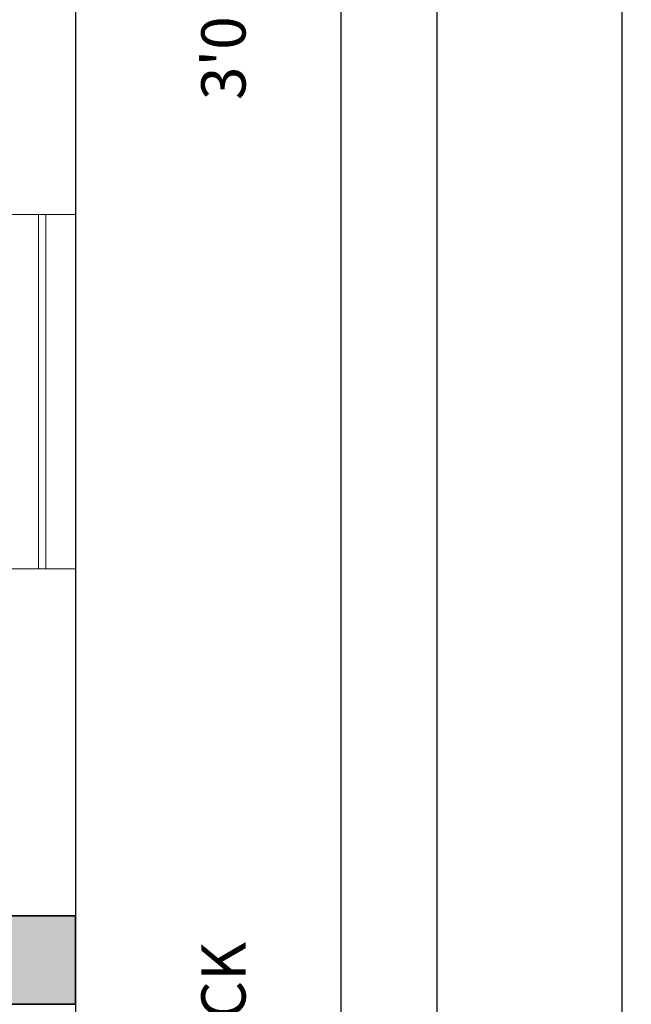
# Model space of a CAD drawing. Units: inches. Extents: x 3321 to 5237, y 11 to 1752.
# Tile 20 of 43: x 4458 to 4541, y 1172 to 1306. Entities that reach past the tile are written whole.
import ezdxf

# ---------------------------------------------------------------- set-up
doc = ezdxf.new("R2010")
doc.units = ezdxf.units.IN
for name, color, linetype, lineweight in [('A-ANNO-DIMS', 2, 'Continuous', 18), ('A-ANNO-TEXT', 7, 'Continuous', 18), ('A-COLS', 1, 'Continuous', 35), ('A-FLOR-EDGE', 7, 'Continuous', 25), ('A-GLAZ', 5, 'Continuous', 18), ('C-PROP', 7, 'Continuous', 30)]:
    doc.layers.add(name, color=color, linetype=linetype, lineweight=lineweight)
doc.styles.get("Standard").update_dxf_attribs({"font": 'arial.ttf'})
doc.dimstyles.new('ISO-25', dxfattribs={"dimtxt": 9, "dimasz": 2.5, "dimexe": 1.25, "dimexo": 0.625, "dimtad": 1, "dimdec": 1, "dimlunit": 3, "dimtxsty": 'Standard', "dimcen": 2.5, "dimclrd": 4, "dimclre": 4, "dimclrt": 256, "dimadec": 0, "dimazin": 0, "dimtfac": 1, "dimtdec": 1, "dimtmove": 0, "dimatfit": 3, "dimfxl": 1, "dimarcsym": 0})

# ---------------------------------------------------------------- blocks, each defined once
blk = doc.blocks.new('*D61')
at = {"layer": 'A-ANNO-DIMS', "color": 0, "lineweight": -2, "transparency": 16777216}
for p, q in [((4502.01, 1687.34), (4515.69, 1687.34)), ((4514.44, 1093.84), (4514.44, 1684.84)), ((4502.01, 1091.34), (4515.69, 1091.34))]:
    blk.add_line(p, q, dxfattribs=at)
at = {"layer": 'A-ANNO-DIMS', "color": 0, "transparency": 16777216}
for points in [[(4514.03, 1684.84), (4514.86, 1684.84), (4514.44, 1687.34)], [(4514.03, 1093.84), (4514.86, 1093.84), (4514.44, 1091.34)]]:
    blk.add_solid(points, dxfattribs=at)
at = {"layer": 'Defpoints', "color": 0, "transparency": 16777216}
for p in [(4501.39, 1687.34), (4514.44, 1687.34), (4501.39, 1091.34)]:
    blk.add_point(p, dxfattribs=at)
at = {"layer": 'A-ANNO-DIMS', "color": 0, "transparency": 16777216, "insert": (4509.22, 1389.34), "char_height": 9, "attachment_point": 5, "rotation": 90}
blk.add_mtext('49\'-8"', dxfattribs=at)
blk = doc.blocks.new('*D64')
at = {"layer": 'A-ANNO-DIMS', "color": 0, "lineweight": -2, "transparency": 16777216}
for p, q in [((4502.01, 1707.34), (4540.73, 1707.34)), ((4539.48, 989.84), (4539.48, 1704.84)), ((4502.01, 987.34), (4540.73, 987.34))]:
    blk.add_line(p, q, dxfattribs=at)
at = {"layer": 'A-ANNO-DIMS', "color": 0, "transparency": 16777216}
for points in [[(4539.06, 1704.84), (4539.9, 1704.84), (4539.48, 1707.34)], [(4539.06, 989.84), (4539.9, 989.84), (4539.48, 987.34)]]:
    blk.add_solid(points, dxfattribs=at)
at = {"layer": 'Defpoints', "color": 0, "transparency": 16777216}
for p in [(4501.39, 1707.34), (4539.48, 1707.34), (4501.39, 987.34)]:
    blk.add_point(p, dxfattribs=at)
at = {"layer": 'A-ANNO-DIMS', "color": 0, "transparency": 16777216, "insert": (4534.26, 1347.34), "char_height": 9, "attachment_point": 5, "rotation": 90}
blk.add_mtext("60'", dxfattribs=at)
blk = doc.blocks.new('COL-9X12-FURN-PLAN')
h = blk.add_hatch(color=256)
h.dxf.hatch_style = 1
h.paths.add_polyline_path([(0, 12), (0, 0), (9, 0), (9, 12)])
blk.add_lwpolyline([(0, 0), (9, 0), (9, 12), (0, 12)], close=True)
blk = doc.blocks.new('WIN-48IN-9IN-WALL')
for p, q in [((0, 0), (0, 9)), ((48, 0), (48, 9)), ((0, 5), (48, 5)), ((0, 4), (48, 4))]:
    blk.add_line(p, q)
blk = doc.blocks.new('PROPERTY-40X60FT')
blk.add_line((0, 720), (0, 0))

msp = doc.modelspace()

# ---------------------------------------------------------------- linework, layer by layer
at = {"layer": 'A-FLOR-EDGE'}
msp.add_line((4465.39, 1687.34), (4465.39, 1091.34), dxfattribs=at)

# ---------------------------------------------------------------- block references
at = {"layer": 'A-COLS'}
msp.add_blockref('COL-9X12-FURN-PLAN', (4456.39, 1172.34), dxfattribs=at)
at = {"layer": 'A-GLAZ', "rotation": 89.99999999999613}
msp.add_blockref('WIN-48IN-9IN-WALL', (4465.39, 1231.34), dxfattribs=at)
at = {"layer": 'C-PROP', "rotation": 180}
msp.add_blockref('PROPERTY-40X60FT', (4501.39, 1707.34), dxfattribs=at)

# ---------------------------------------------------------------- texts
at = {"layer": 'A-ANNO-TEXT', "char_height": 6, "attachment_point": 1, "rotation": 90}
for insert in [(4482.45, 1294.84), (4482.45, 1128.26)]:
    msp.add_mtext_dynamic_manual_height_columns('3\'0" SETBACK', width=97.3114, gutter_width=25, heights=[0], dxfattribs=dict(at, insert=insert))

# ---------------------------------------------------------------- dimensions: what is measured, and where the dimension line sits
at = {"layer": 'A-ANNO-DIMS'}
for base, p1, p2, angle, override, picture, middle in [((4539.48, 1707.34), (4501.39, 987.34), (4501.39, 1707.34), 270, {"dimclrd": 0, "dimclre": 0, "dimclrt": 0}, '*D64', (4534.26, 1347.34)), ((4514.44, 1687.34), (4501.39, 1091.34), (4501.39, 1687.34), 90, {"dimclrd": 0, "dimclre": 0, "dimclrt": 0, "dimtmove": 1}, '*D61', (4509.22, 1389.34))]:
    dim = msp.add_linear_dim(base=base, p1=p1, p2=p2, angle=angle, dimstyle='ISO-25', override=override, dxfattribs=at)
    dim.commit()
    dim.dimension.update_dxf_attribs({"geometry": picture, "text_midpoint": middle})

doc.saveas('drawing.dxf')
